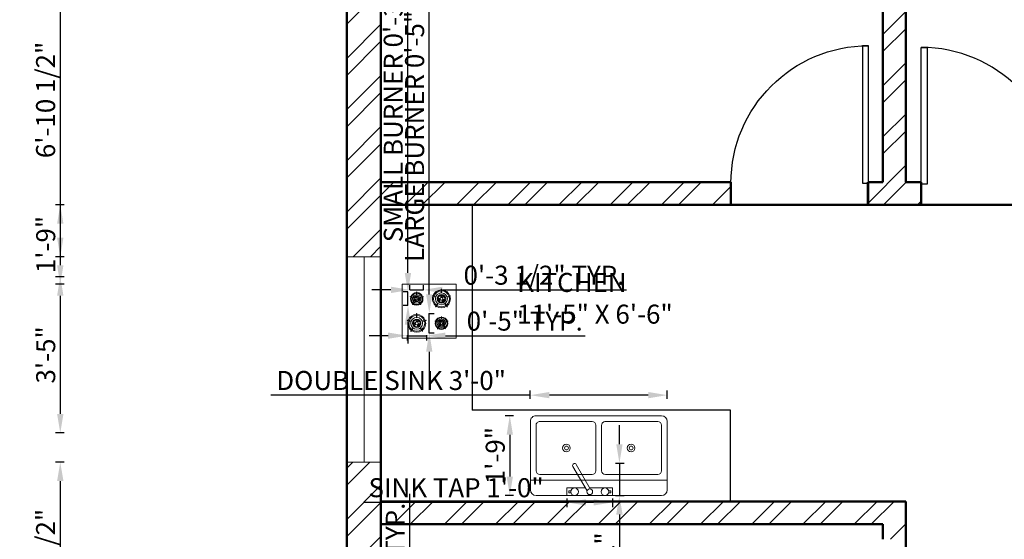
# Model space of a CAD drawing. Units: inches. Extents: x -83 to 371, y -457 to 76.
# Tile 2 of 4: x -83 to 176, y -243 to -107. Entities that reach past the tile are written whole.
import ezdxf

# ---------------------------------------------------------------- set-up
doc = ezdxf.new("R2010")
doc.units = ezdxf.units.IN
for name, color, linetype, lineweight in [('A-ANNO-DIMS', 2, 'Continuous', 18), ('A-AREA-IDEN', 7, 'Continuous', 25), ('A-DOOR', 3, 'Continuous', 25), ('A-EQPM', 8, 'Continuous', 18), ('A-FLOR-CASE', 8, 'Continuous', 25), ('A-FLOR-FIXT', 9, 'Continuous', 18), ('A-GLAZ', 4, 'Continuous', 18), ('A-WALL', 7, 'Continuous', 50), ('A-WALL-PATT', 252, 'Continuous', 13)]:
    doc.layers.add(name, color=color, linetype=linetype, lineweight=lineweight)
doc.styles.get("Standard").update_dxf_attribs({"font": 'arial.ttf'})
doc.dimstyles.new('ISO-25', dxfattribs={"dimtxt": 5, "dimasz": 5, "dimexe": 1.25, "dimexo": 0.625, "dimtad": 1, "dimlunit": 3, "dimtxsty": 'Standard', "dimcen": 2.5, "dimadec": 0, "dimazin": 0, "dimtfac": 1, "dimtmove": 0, "dimatfit": 3, "dimfxl": 1, "dimfxlon": 1, "dimarcsym": 0})

# ---------------------------------------------------------------- blocks, each defined once
blk = doc.blocks.new('*U4')
for p, q in [((0, 0), (0, -6)), ((40, 0), (40, -6))]:
    blk.add_line(p, q)
blk.add_lwpolyline([(0, 0), (0, 40), (1.75, 40), (1.75, 0)], close=True)
blk.add_arc((0, 0), 40, 0, 90)
blk = doc.blocks.new('Sink-double - 36 in top')
for p, q in [((-18, -4), (18, -4)), ((-0.75, -18.5), (-0.75, -6.5)), ((0.75, -6.5), (0.75, -18.5))]:
    blk.add_line(p, q)
for points in [[(-16.5, 0), (16.5, 0)], [(-18, -19.5), (-18, -1.5)], [(18, -1.5), (18, -19.5)], [(-16.5, -18.5), (-16.5, -6.5)], [(-15.5, -5.5), (-1.75, -5.5)], [(1.75, -5.5), (15.5, -5.5)], [(16.5, -6.5), (16.5, -18.5)], [(-1.75, -19.5), (-15.5, -19.5)], [(15.5, -19.5), (1.75, -19.5)], [(16.5, -21), (-16.5, -21)]]:
    blk.add_lwpolyline(points)
for centre, radius in [((-8.5, -12.5), 1), ((-8.5, -12.5), 0.5), ((8.5, -12.5), 1), ((8.5, -12.5), 0.5)]:
    blk.add_circle(centre, radius)
for centre, radius, start, end in [((-16.5, -1.5), 1.5, 90, 180), ((16.5, -1.5), 1.5, 0, 90), ((-15.5, -6.5), 1, 90, 180), ((-1.75, -6.5), 1, 0, 90), ((1.75, -6.5), 1, 90, 180), ((15.5, -6.5), 1, 0, 90), ((-16.5, -19.5), 1.5, 180, 270), ((-15.5, -18.5), 1, 180, 270), ((-1.75, -18.5), 1, 270, 0), ((1.75, -18.5), 1, 180, 270), ((15.5, -18.5), 1, 270, 0), ((16.5, -19.5), 1.5, 270, 0)]:
    blk.add_arc(centre, radius, start, end)
blk = doc.blocks.new('Faucet - kit sink top')
for p, q in [((-5.5, -0.75), (-5.5, -1.25)), ((-4.94278, -0.75), (-5.5, -0.75)), ((-5.5, -1.25), (-4.94278, -1.25)), ((-0.14775, -1.7441), (3.56698, -8.1782)), ((4.43301, -7.6782), (0.71828, -1.2441)), ((4.94278, -0.75), (5.5, -0.75)), ((5.5, -1.25), (4.94278, -1.25)), ((5.5, -0.75), (5.5, -1.25))]:
    blk.add_line(p, q)
blk.add_lwpolyline([(-0.00587, -2), (-6, -2), (-6, 0), (6, 0), (6, -2), (1.15195, -2)])
for centre, radius in [((-4, -1), 1), ((4, -1), 1), ((0, -1), 0.75)]:
    blk.add_circle(centre, radius)
blk.add_arc((4, -7.9282), 0.5, 210, 30)
blk = doc.blocks.new('WIN-54IN')
blk.add_line((4.5, 54), (4.5, 0))
blk.add_lwpolyline([(0, 54), (9, 54), (9, 0), (0, 0)], close=True)
blk = doc.blocks.new('COOKTOP-BURNER-LARGE')
for p, q in [((0.94, 2.8), (0.03, 3.1)), ((0.97, 2.88), (0.05, 3.18)), ((2.44, 3.95), (2.44, 4.91)), ((2.52, 3.95), (2.52, 4.91)), ((3.99, 2.88), (4.91, 3.18)), ((4.02, 2.8), (4.93, 3.1)), ((1.51, 1.07), (0.94, 0.29)), ((1.57, 1.03), (1, 0.25)), ((3.39, 1.03), (3.96, 0.25)), ((3.45, 1.07), (4.02, 0.29))]:
    blk.add_line(p, q)
for radius in [1.56, 1.12, 0.912, 0.391]:
    blk.add_circle((2.48, 2.35), radius)
for centre, radius, start, end in [((0.04, 3.14), 0.0391, 72.0007, 252.0007), ((2.48, 2.35), 2.35, 162.9557, 233.0457), ((2.48, 2.35), 2.35, 90.9557, 161.0457), ((2.48, 2.35), 2.09, 163.075, 232.9263), ((2.48, 2.35), 2.09, 91.075, 160.9263), ((0.95, 2.84), 0.0391, 252.0007, 72.0007), ((2.44, 3), 0.13, 93.5265, 273.5265), ((2.48, 2.35), 0.782, 60.0007, 93.5265), ((2.48, 4.91), 0.0391, 0.0007, 180.0007), ((2.48, 3.95), 0.0391, 180.0007, 0.0007), ((2.48, 2.35), 0.521, 60.0007, 93.5265), ((2.48, 2.35), 2.35, 18.9557, 89.0457), ((2.48, 2.35), 2.09, 19.075, 88.9263), ((2.81, 2.91), 0.13, 240.0007, 60.0007), ((2.48, 2.35), 2.09, 307.075, 16.9263), ((2.48, 2.35), 2.35, 306.9557, 17.0457), ((4, 2.84), 0.0391, 108.0007, 288.0007), ((4.92, 3.14), 0.0391, 288.0007, 108.0007), ((0.97, 0.27), 0.0391, 144.0007, 324.0007), ((2.48, 2.35), 2.35, 234.9557, 305.0457), ((2.48, 2.35), 2.09, 235.075, 304.9263), ((1.54, 1.05), 0.0391, 324.0007, 144.0007), ((1.83, 2.35), 0.13, 0.0007, 180.0007), ((2.48, 2.35), 0.782, 180.0007, 213.5265), ((1.94, 1.99), 0.13, 213.5265, 33.5265), ((2.48, 2.35), 0.521, 180.0007, 213.5265), ((2.81, 1.78), 0.13, 120.0007, 300.0007), ((2.48, 2.35), 0.521, 300.0007, 333.5265), ((2.48, 2.35), 0.782, 300.0007, 333.5265), ((3.06, 2.06), 0.13, 333.5265, 153.5265), ((3.42, 1.05), 0.0391, 36.0007, 216.0007), ((3.99, 0.27), 0.0391, 216.0007, 36.0007)]:
    blk.add_arc(centre, radius, start, end)
blk = doc.blocks.new('COOKTOP-BURNER-SMALL')
for p, q in [((1.71, 2.77), (1.71, 3.44)), ((1.76, 2.77), (1.76, 3.44)), ((0.66, 1.96), (0.02, 2.17)), ((0.68, 2.02), (0.04, 2.22)), ((1.05, 0.75), (0.66, 0.21)), ((1.1, 0.72), (0.7, 0.17)), ((2.37, 0.72), (2.77, 0.17)), ((2.42, 0.75), (2.81, 0.21)), ((2.79, 2.02), (3.44, 2.22)), ((2.81, 1.96), (3.45, 2.17))]:
    blk.add_line(p, q)
for radius in [1.09, 0.785, 0.639, 0.274]:
    blk.add_circle((1.74, 1.64), radius)
for centre, radius, start, end in [((1.74, 1.64), 1.64, 90.9557, 161.0457), ((1.74, 1.64), 1.46, 91.075, 160.9263), ((1.74, 3.44), 0.0274, 0.0007, 180.0007), ((1.74, 2.77), 0.0274, 180.0007, 0.0007), ((1.74, 1.64), 1.64, 18.9557, 89.0457), ((1.74, 1.64), 1.46, 19.075, 88.9263), ((0.03, 2.2), 0.0274, 72.0007, 252.0007), ((1.74, 1.64), 1.64, 162.9557, 233.0457), ((1.74, 1.64), 1.46, 163.075, 232.9263), ((0.68, 0.19), 0.0274, 144.0007, 324.0007), ((0.67, 1.99), 0.0274, 252.0007, 72.0007), ((1.67, 1.64), 1.64, 234.9557, 305.0457), ((1.74, 1.64), 1.46, 235.075, 304.9263), ((1.08, 0.73), 0.0274, 324.0007, 144.0007), ((1.33, 1.44), 0.0912, 26.4748, 206.4748), ((1.74, 1.64), 0.547, 206.4748, 240.0007), ((1.74, 1.64), 0.365, 206.4748, 240.0007), ((1.51, 2.04), 0.0912, 120.0007, 300.0007), ((1.74, 1.64), 0.547, 86.4748, 120.0007), ((1.51, 1.25), 0.0912, 240.0007, 60.0007), ((1.74, 1.64), 0.365, 86.4748, 120.0007), ((1.76, 2.1), 0.0912, 266.4748, 86.4748), ((2.12, 1.39), 0.0912, 146.4748, 326.4748), ((1.74, 1.64), 0.365, 326.4748, 0.0007), ((2.19, 1.64), 0.0912, 0.0007, 180.0007), ((1.74, 1.64), 0.547, 326.4748, 0.0007), ((2.4, 0.73), 0.0274, 36.0007, 216.0007), ((1.74, 1.64), 1.46, 307.075, 16.9263), ((1.74, 1.64), 1.64, 306.9557, 17.0457), ((2.79, 0.19), 0.0274, 216.0007, 36.0007), ((2.8, 1.99), 0.0274, 108.0007, 288.0007), ((3.44, 2.2), 0.0274, 288.0007, 108.0007)]:
    blk.add_arc(centre, radius, start, end)
blk = doc.blocks.new('*D24')
at = {"layer": 'A-ANNO-DIMS', "color": 0, "lineweight": -2, "transparency": 16777216}
for p, q in [((19.57, -332.63), (19.57, -231.32)), ((20.57, -332.63), (18.32, -332.63)), ((19.57, -344.37), (19.57, -337.63)), ((20.57, -349.37), (18.32, -349.37))]:
    blk.add_line(p, q, dxfattribs=at)
at = {"layer": 'A-ANNO-DIMS', "color": 0, "transparency": 16777216}
for points in [[(18.74, -337.63), (20.4, -337.63), (19.57, -332.63)], [(18.74, -344.37), (20.4, -344.37), (19.57, -349.37)]]:
    blk.add_solid(points, dxfattribs=at)
at = {"layer": 'Defpoints', "color": 0, "transparency": 16777216}
for p in [(19.57, -332.63), (22.08, -332.63), (22.08, -349.37)]:
    blk.add_point(p, dxfattribs=at)
at = {"layer": 'A-ANNO-DIMS', "color": 0, "transparency": 16777216, "insert": (16.36, -279.48), "char_height": 5, "attachment_point": 5, "rotation": 90}
blk.add_mtext('NIGHTSTAND L 1\'-4 1/2" TYP.', dxfattribs=at)
blk = doc.blocks.new('*D30')
at = {"layer": 'A-ANNO-DIMS', "color": 0, "lineweight": -2, "transparency": 16777216}
for p, q in [((24.67, -178.88), (24.67, -85.32)), ((24.53, -183.88), (25.92, -183.88)), ((24.67, -188.98), (24.67, -183.88)), ((24.53, -188.98), (25.92, -188.98)), ((24.67, -193.98), (24.67, -198.98))]:
    blk.add_line(p, q, dxfattribs=at)
at = {"layer": 'A-ANNO-DIMS', "color": 0, "transparency": 16777216}
for points in [[(23.83, -178.88), (25.5, -178.88), (24.67, -183.88)], [(23.83, -193.98), (25.5, -193.98), (24.67, -188.98)]]:
    blk.add_solid(points, dxfattribs=at)
at = {"layer": 'Defpoints', "color": 0, "transparency": 16777216}
for p in [(23.9, -183.88), (24.67, -183.88), (23.9, -188.98)]:
    blk.add_point(p, dxfattribs=at)
at = {"layer": 'A-ANNO-DIMS', "color": 0, "transparency": 16777216, "insert": (21.46, -129.6), "char_height": 5, "attachment_point": 5, "rotation": 90}
blk.add_mtext('LARGE BURNER 0\'-5" TYP.', dxfattribs=at)
blk = doc.blocks.new('*D31')
at = {"layer": 'A-ANNO-DIMS', "color": 0, "lineweight": -2, "transparency": 16777216}
for p, q in [((13.84, -189.74), (8.84, -189.74)), ((18.84, -189.6), (18.84, -190.99)), ((18.84, -189.74), (23.9, -189.74)), ((23.9, -189.6), (23.9, -190.99)), ((28.9, -189.74), (65.63, -189.74))]:
    blk.add_line(p, q, dxfattribs=at)
at = {"layer": 'A-ANNO-DIMS', "color": 0, "transparency": 16777216}
for points in [[(13.84, -188.91), (13.84, -190.57), (18.84, -189.74)], [(28.9, -188.91), (28.9, -190.57), (23.9, -189.74)]]:
    blk.add_solid(points, dxfattribs=at)
at = {"layer": 'Defpoints', "color": 0, "transparency": 16777216}
for p in [(18.84, -188.98), (23.9, -188.98), (23.9, -189.74)]:
    blk.add_point(p, dxfattribs=at)
at = {"layer": 'A-ANNO-DIMS', "color": 0, "transparency": 16777216, "insert": (49.77, -186.56), "char_height": 5, "attachment_point": 5}
blk.add_mtext('0\'-5" TYP.', dxfattribs=at)
blk = doc.blocks.new('*D32')
at = {"layer": 'A-ANNO-DIMS', "color": 0, "lineweight": -2, "transparency": 16777216}
for p, q in [((19.06, -173.23), (19.06, -68.59)), ((19.06, -178.23), (17.81, -178.23)), ((19.06, -181.8), (19.06, -178.23)), ((19.06, -181.8), (17.81, -181.8)), ((19.06, -186.8), (19.06, -191.8))]:
    blk.add_line(p, q, dxfattribs=at)
at = {"layer": 'A-ANNO-DIMS', "color": 0, "transparency": 16777216}
for points in [[(18.23, -173.23), (19.9, -173.23), (19.06, -178.23)], [(18.23, -186.8), (19.9, -186.8), (19.06, -181.8)]]:
    blk.add_solid(points, dxfattribs=at)
at = {"layer": 'Defpoints', "color": 0, "transparency": 16777216}
for p in [(19.06, -178.23), (19.6, -178.23), (19.6, -181.8)]:
    blk.add_point(p, dxfattribs=at)
at = {"layer": 'A-ANNO-DIMS', "color": 0, "transparency": 16777216, "insert": (15.85, -118.41), "char_height": 5, "attachment_point": 5, "rotation": 90}
blk.add_mtext('SMALL BURNER 0\'-3 1/2" TYP.', dxfattribs=at)
blk = doc.blocks.new('*D33')
at = {"layer": 'A-ANNO-DIMS', "color": 0, "lineweight": -2, "transparency": 16777216}
for p, q in [((14.6, -177.7), (9.6, -177.7)), ((19.6, -177.7), (19.6, -176.45)), ((19.6, -177.7), (23.14, -177.7)), ((23.14, -177.7), (23.14, -176.45)), ((28.14, -177.7), (76.52, -177.7))]:
    blk.add_line(p, q, dxfattribs=at)
at = {"layer": 'A-ANNO-DIMS', "color": 0, "transparency": 16777216}
for points in [[(14.6, -176.86), (14.6, -178.53), (19.6, -177.7)], [(28.14, -176.86), (28.14, -178.53), (23.14, -177.7)]]:
    blk.add_solid(points, dxfattribs=at)
at = {"layer": 'Defpoints', "color": 0, "transparency": 16777216}
for p in [(19.6, -178.23), (23.14, -177.7), (23.14, -178.23)]:
    blk.add_point(p, dxfattribs=at)
at = {"layer": 'A-ANNO-DIMS', "color": 0, "transparency": 16777216, "insert": (54.83, -174.48), "char_height": 5, "attachment_point": 5}
blk.add_mtext('0\'-3 1/2" TYP.', dxfattribs=at)
blk = doc.blocks.new('*D34')
at = {"layer": 'A-ANNO-DIMS', "color": 0, "lineweight": -2, "transparency": 16777216}
for p, q in [((51.24, -206.38), (51.24, -204.13)), ((87.24, -206.38), (87.24, -204.13)), ((51.24, -205.38), (-16.96, -205.38)), ((82.24, -205.38), (56.24, -205.38))]:
    blk.add_line(p, q, dxfattribs=at)
at = {"layer": 'A-ANNO-DIMS', "color": 0, "transparency": 16777216}
for points in [[(56.24, -204.55), (56.24, -206.21), (51.24, -205.38)], [(82.24, -204.55), (82.24, -206.21), (87.24, -205.38)]]:
    blk.add_solid(points, dxfattribs=at)
at = {"layer": 'Defpoints', "color": 0, "transparency": 16777216}
for p in [(51.24, -205.38), (51.24, -210.78), (87.24, -210.78)]:
    blk.add_point(p, dxfattribs=at)
at = {"layer": 'A-ANNO-DIMS', "color": 0, "transparency": 16777216, "insert": (14.64, -202.17), "char_height": 5, "attachment_point": 5}
blk.add_mtext('DOUBLE SINK 3\'-0"', dxfattribs=at)
blk = doc.blocks.new('*D35')
at = {"layer": 'A-ANNO-DIMS', "color": 0, "lineweight": -2, "transparency": 16777216}
for p, q in [((46.84, -210.78), (44.59, -210.78)), ((45.84, -215.78), (45.84, -226.78)), ((46.84, -231.78), (44.59, -231.78))]:
    blk.add_line(p, q, dxfattribs=at)
at = {"layer": 'A-ANNO-DIMS', "color": 0, "transparency": 16777216}
for points in [[(45.01, -215.78), (46.67, -215.78), (45.84, -210.78)], [(45.01, -226.78), (46.67, -226.78), (45.84, -231.78)]]:
    blk.add_solid(points, dxfattribs=at)
at = {"layer": 'Defpoints', "color": 0, "transparency": 16777216}
for p in [(51.24, -210.78), (45.84, -231.78), (51.24, -231.78)]:
    blk.add_point(p, dxfattribs=at)
at = {"layer": 'A-ANNO-DIMS', "color": 0, "transparency": 16777216, "insert": (42.66, -221.28), "char_height": 5, "attachment_point": 5, "rotation": 90}
blk.add_mtext('1\'-9"', dxfattribs=at)
blk = doc.blocks.new('*D36')
at = {"layer": 'A-ANNO-DIMS', "color": 0, "lineweight": -2, "transparency": 16777216}
for p, q in [((60.86, -232.58), (60.86, -234.83)), ((72.86, -232.58), (72.86, -234.83)), ((60.86, -233.58), (7.58, -233.58)), ((67.86, -233.58), (65.86, -233.58))]:
    blk.add_line(p, q, dxfattribs=at)
at = {"layer": 'A-ANNO-DIMS', "color": 0, "transparency": 16777216}
for points in [[(65.86, -232.75), (65.86, -234.41), (60.86, -233.58)], [(67.86, -232.75), (67.86, -234.41), (72.86, -233.58)]]:
    blk.add_solid(points, dxfattribs=at)
at = {"layer": 'Defpoints', "color": 0, "transparency": 16777216}
for p in [(60.86, -231.78), (72.86, -231.78), (60.86, -233.58)]:
    blk.add_point(p, dxfattribs=at)
at = {"layer": 'A-ANNO-DIMS', "color": 0, "transparency": 16777216, "insert": (31.72, -230.37), "char_height": 5, "attachment_point": 5}
blk.add_mtext('SINK TAP 1\'-0"', dxfattribs=at)
blk = doc.blocks.new('*D37')
at = {"layer": 'A-ANNO-DIMS', "color": 0, "lineweight": -2, "transparency": 16777216}
for p, q in [((74.66, -218.28), (74.66, -213.28)), ((73.66, -223.28), (75.91, -223.28)), ((74.66, -223.28), (74.66, -231.78)), ((73.66, -231.78), (75.91, -231.78)), ((74.66, -236.78), (74.66, -267.97))]:
    blk.add_line(p, q, dxfattribs=at)
at = {"layer": 'A-ANNO-DIMS', "color": 0, "transparency": 16777216}
for points in [[(73.83, -218.28), (75.5, -218.28), (74.66, -223.28)], [(73.83, -236.78), (75.5, -236.78), (74.66, -231.78)]]:
    blk.add_solid(points, dxfattribs=at)
at = {"layer": 'Defpoints', "color": 0, "transparency": 16777216}
for p in [(72.86, -223.28), (72.86, -231.78), (74.66, -231.78)]:
    blk.add_point(p, dxfattribs=at)
at = {"layer": 'A-ANNO-DIMS', "color": 0, "transparency": 16777216, "insert": (71.45, -254.88), "char_height": 5, "attachment_point": 5, "rotation": 90}
blk.add_mtext('0\'-8 1/2"', dxfattribs=at)
blk = doc.blocks.new('*D39')
at = {"layer": 'A-ANNO-DIMS', "color": 0, "lineweight": -2, "transparency": 16777216}
for p, q in [((-71.36, -86.5), (-73.61, -86.5)), ((-72.36, -91.5), (-72.36, -163.99)), ((-71.36, -168.99), (-73.61, -168.99))]:
    blk.add_line(p, q, dxfattribs=at)
at = {"layer": 'A-ANNO-DIMS', "color": 0, "transparency": 16777216}
for points in [[(-73.19, -91.5), (-71.52, -91.5), (-72.36, -86.5)], [(-73.19, -163.99), (-71.52, -163.99), (-72.36, -168.99)]]:
    blk.add_solid(points, dxfattribs=at)
at = {"layer": 'Defpoints', "color": 0, "transparency": 16777216}
for p in [(2.94, -86.5), (-72.36, -168.99), (3.06, -168.99)]:
    blk.add_point(p, dxfattribs=at)
at = {"layer": 'A-ANNO-DIMS', "color": 0, "transparency": 16777216, "insert": (-75.57, -127.74), "char_height": 5, "attachment_point": 5, "rotation": 90}
blk.add_mtext('6\'-10 1/2"', dxfattribs=at)
blk = doc.blocks.new('*D40')
at = {"layer": 'A-ANNO-DIMS', "color": 0, "lineweight": -2, "transparency": 16777216}
for p, q in [((-71.36, -222.99), (-73.61, -222.99)), ((-72.36, -227.99), (-72.36, -269.39)), ((-71.36, -274.39), (-73.61, -274.39))]:
    blk.add_line(p, q, dxfattribs=at)
at = {"layer": 'A-ANNO-DIMS', "color": 0, "transparency": 16777216}
for points in [[(-73.19, -227.99), (-71.52, -227.99), (-72.36, -222.99)], [(-73.19, -269.39), (-71.52, -269.39), (-72.36, -274.39)]]:
    blk.add_solid(points, dxfattribs=at)
at = {"layer": 'Defpoints', "color": 0, "transparency": 16777216}
for p in [(3.06, -222.99), (-72.36, -274.39), (3.85, -274.39)]:
    blk.add_point(p, dxfattribs=at)
at = {"layer": 'A-ANNO-DIMS', "color": 0, "transparency": 16777216, "insert": (-75.57, -248.69), "char_height": 5, "attachment_point": 5, "rotation": 90}
blk.add_mtext('4\'-3 1/2"', dxfattribs=at)
blk = doc.blocks.new('*D45')
at = {"layer": 'A-ANNO-DIMS', "color": 0, "lineweight": -2, "transparency": 16777216}
for p, q in [((143.97, -455.2), (143.97, -457.45)), ((149.97, -455.2), (149.97, -457.45)), ((138.97, -456.2), (133.97, -456.2)), ((143.97, -456.2), (149.97, -456.2)), ((154.97, -456.2), (174.51, -456.2))]:
    blk.add_line(p, q, dxfattribs=at)
at = {"layer": 'A-ANNO-DIMS', "color": 0, "transparency": 16777216}
for points in [[(138.97, -455.37), (138.97, -457.03), (143.97, -456.2)], [(154.97, -455.37), (154.97, -457.03), (149.97, -456.2)]]:
    blk.add_solid(points, dxfattribs=at)
at = {"layer": 'Defpoints', "color": 0, "transparency": 16777216}
for p in [(143.97, 6.68), (149.97, 6.68), (149.97, -456.2)]:
    blk.add_point(p, dxfattribs=at)
at = {"layer": 'A-ANNO-DIMS', "color": 0, "transparency": 16777216, "insert": (167.24, -453.02), "char_height": 5, "attachment_point": 5}
blk.add_mtext('0\'-6"', dxfattribs=at)
blk = doc.blocks.new('*D46')
at = {"layer": 'A-ANNO-DIMS', "color": 0, "lineweight": -2, "transparency": 16777216}
for p, q in [((103.97, 39.58), (103.97, 41.83)), ((139.97, 39.58), (139.97, 41.83)), ((108.97, 40.58), (134.97, 40.58))]:
    blk.add_line(p, q, dxfattribs=at)
at = {"layer": 'A-ANNO-DIMS', "color": 0, "transparency": 16777216}
for points in [[(108.97, 41.41), (108.97, 39.74), (103.97, 40.58)], [(134.97, 41.41), (134.97, 39.74), (139.97, 40.58)]]:
    blk.add_solid(points, dxfattribs=at)
at = {"layer": 'Defpoints', "color": 0, "transparency": 16777216}
for p in [(139.97, 40.58), (103.97, -149.32), (139.97, -149.32)]:
    blk.add_point(p, dxfattribs=at)
at = {"layer": 'A-ANNO-DIMS', "color": 0, "transparency": 16777216, "insert": (121.97, 43.75), "char_height": 5, "attachment_point": 5}
blk.add_mtext('3\'-0"', dxfattribs=at)
blk = doc.blocks.new('*D47')
at = {"layer": 'A-ANNO-DIMS', "color": 0, "lineweight": -2, "transparency": 16777216}
for p, q in [((139.97, 39.58), (139.97, 41.83)), ((143.97, 39.58), (143.97, 41.83)), ((134.97, 40.58), (129.97, 40.58)), ((139.97, 40.58), (143.97, 40.58)), ((148.97, 40.58), (168.51, 40.58))]:
    blk.add_line(p, q, dxfattribs=at)
at = {"layer": 'A-ANNO-DIMS', "color": 0, "transparency": 16777216}
for points in [[(134.97, 41.41), (134.97, 39.74), (139.97, 40.58)], [(148.97, 41.41), (148.97, 39.74), (143.97, 40.58)]]:
    blk.add_solid(points, dxfattribs=at)
at = {"layer": 'Defpoints', "color": 0, "transparency": 16777216}
for p in [(143.97, 40.58), (139.97, -149.32), (143.97, -149.32)]:
    blk.add_point(p, dxfattribs=at)
at = {"layer": 'A-ANNO-DIMS', "color": 0, "transparency": 16777216, "insert": (161.24, 43.75), "char_height": 5, "attachment_point": 5}
blk.add_mtext('0\'-4"', dxfattribs=at)
blk = doc.blocks.new('*D55')
at = {"layer": 'A-ANNO-DIMS', "color": 0, "lineweight": -2, "transparency": 16777216}
for p, q in [((11.97, -455.2), (11.97, -457.45)), ((103.87, -455.2), (103.87, -457.45)), ((16.97, -456.2), (98.87, -456.2))]:
    blk.add_line(p, q, dxfattribs=at)
at = {"layer": 'A-ANNO-DIMS', "color": 0, "transparency": 16777216}
for points in [[(16.97, -455.37), (16.97, -457.03), (11.97, -456.2)], [(98.87, -455.37), (98.87, -457.03), (103.87, -456.2)]]:
    blk.add_solid(points, dxfattribs=at)
at = {"layer": 'Defpoints', "color": 0, "transparency": 16777216}
for p in [(11.97, -233.32), (103.87, -233.32), (103.87, -456.2)]:
    blk.add_point(p, dxfattribs=at)
at = {"layer": 'A-ANNO-DIMS', "color": 0, "transparency": 16777216, "insert": (57.92, -453.02), "char_height": 5, "attachment_point": 5}
blk.add_mtext('7\'-8"', dxfattribs=at)
blk = doc.blocks.new('*D56')
at = {"layer": 'A-ANNO-DIMS', "color": 0, "lineweight": -2, "transparency": 16777216}
for p, q in [((365.66, -209.32), (367.91, -209.32)), ((366.66, -228.32), (366.66, -214.32)), ((365.66, -233.32), (367.91, -233.32))]:
    blk.add_line(p, q, dxfattribs=at)
at = {"layer": 'A-ANNO-DIMS', "color": 0, "transparency": 16777216}
for points in [[(365.83, -214.32), (367.49, -214.32), (366.66, -209.32)], [(365.83, -228.32), (367.49, -228.32), (366.66, -233.32)]]:
    blk.add_solid(points, dxfattribs=at)
at = {"layer": 'Defpoints', "color": 0, "transparency": 16777216}
for p in [(103.87, -209.32), (366.66, -209.32), (103.87, -233.32)]:
    blk.add_point(p, dxfattribs=at)
at = {"layer": 'A-ANNO-DIMS', "color": 0, "transparency": 16777216, "insert": (363.48, -221.32), "char_height": 5, "attachment_point": 5, "rotation": 90}
blk.add_mtext('2\'-0"', dxfattribs=at)
blk = doc.blocks.new('*D57')
at = {"layer": 'A-ANNO-DIMS', "color": 0, "lineweight": -2, "transparency": 16777216}
for p, q in [((365.66, -155.32), (367.91, -155.32)), ((366.66, -160.32), (366.66, -204.32)), ((365.66, -209.32), (367.91, -209.32))]:
    blk.add_line(p, q, dxfattribs=at)
at = {"layer": 'A-ANNO-DIMS', "color": 0, "transparency": 16777216}
for points in [[(365.83, -160.32), (367.49, -160.32), (366.66, -155.32)], [(365.83, -204.32), (367.49, -204.32), (366.66, -209.32)]]:
    blk.add_solid(points, dxfattribs=at)
at = {"layer": 'Defpoints', "color": 0, "transparency": 16777216}
for p in [(35.97, -155.32), (35.97, -209.32), (366.66, -209.32)]:
    blk.add_point(p, dxfattribs=at)
at = {"layer": 'A-ANNO-DIMS', "color": 0, "transparency": 16777216, "insert": (363.48, -182.32), "char_height": 5, "attachment_point": 5, "rotation": 90}
blk.add_mtext('4\'-6"', dxfattribs=at)
blk = doc.blocks.new('*D58')
at = {"layer": 'A-ANNO-DIMS', "color": 0, "lineweight": -2, "transparency": 16777216}
for p, q in [((11.97, 39.58), (11.97, 41.83)), ((35.97, 39.58), (35.97, 41.83)), ((16.97, 40.58), (30.97, 40.58))]:
    blk.add_line(p, q, dxfattribs=at)
at = {"layer": 'A-ANNO-DIMS', "color": 0, "transparency": 16777216}
for points in [[(16.97, 41.41), (16.97, 39.74), (11.97, 40.58)], [(30.97, 41.41), (30.97, 39.74), (35.97, 40.58)]]:
    blk.add_solid(points, dxfattribs=at)
at = {"layer": 'Defpoints', "color": 0, "transparency": 16777216}
for p in [(35.97, 40.58), (11.97, -155.32), (35.97, -155.32)]:
    blk.add_point(p, dxfattribs=at)
at = {"layer": 'A-ANNO-DIMS', "color": 0, "transparency": 16777216, "insert": (23.97, 43.75), "char_height": 5, "attachment_point": 5}
blk.add_mtext('2\'-0"', dxfattribs=at)
blk = doc.blocks.new('*D59')
at = {"layer": 'A-ANNO-DIMS', "color": 0, "lineweight": -2, "transparency": 16777216}
for p, q in [((17.51, 39.58), (17.51, 41.83)), ((31.73, 39.58), (31.73, 41.83)), ((22.51, 40.58), (26.73, 40.58))]:
    blk.add_line(p, q, dxfattribs=at)
at = {"layer": 'A-ANNO-DIMS', "color": 0, "transparency": 16777216}
for points in [[(22.51, 41.41), (22.51, 39.74), (17.51, 40.58)], [(26.73, 41.41), (26.73, 39.74), (31.73, 40.58)]]:
    blk.add_solid(points, dxfattribs=at)
at = {"layer": 'Defpoints', "color": 0, "transparency": 16777216}
for p in [(31.73, 40.58), (17.51, -176.2), (31.73, -176.2)]:
    blk.add_point(p, dxfattribs=at)
at = {"layer": 'A-ANNO-DIMS', "color": 0, "transparency": 16777216, "insert": (24.62, 43.71), "char_height": 5, "attachment_point": 5}
blk.add_mtext('1\'-2"', dxfattribs=at)
blk = doc.blocks.new('*D60')
at = {"layer": 'A-ANNO-DIMS', "color": 0, "lineweight": -2, "transparency": 16777216}
for p, q in [((365.66, -176.2), (367.91, -176.2)), ((366.66, -181.2), (366.66, -185.42)), ((365.66, -190.42), (367.91, -190.42))]:
    blk.add_line(p, q, dxfattribs=at)
at = {"layer": 'A-ANNO-DIMS', "color": 0, "transparency": 16777216}
for points in [[(365.83, -181.2), (367.49, -181.2), (366.66, -176.2)], [(365.83, -185.42), (367.49, -185.42), (366.66, -190.42)]]:
    blk.add_solid(points, dxfattribs=at)
at = {"layer": 'Defpoints', "color": 0, "transparency": 16777216}
for p in [(31.73, -176.2), (31.73, -190.42), (366.66, -190.42)]:
    blk.add_point(p, dxfattribs=at)
at = {"layer": 'A-ANNO-DIMS', "color": 0, "transparency": 16777216, "insert": (363.52, -183.31), "char_height": 5, "attachment_point": 5, "rotation": 90}
blk.add_mtext('1\'-2"', dxfattribs=at)
blk = doc.blocks.new('*D62')
at = {"layer": 'A-ANNO-DIMS', "color": 0, "lineweight": -2, "transparency": 16777216}
for p, q in [((-71.36, -174.24), (-73.61, -174.24)), ((-72.36, -179.24), (-72.36, -210.33)), ((-71.36, -215.33), (-73.61, -215.33))]:
    blk.add_line(p, q, dxfattribs=at)
at = {"layer": 'A-ANNO-DIMS', "color": 0, "transparency": 16777216}
for points in [[(-73.19, -179.24), (-71.52, -179.24), (-72.36, -174.24)], [(-73.19, -210.33), (-71.52, -210.33), (-72.36, -215.33)]]:
    blk.add_solid(points, dxfattribs=at)
at = {"layer": 'Defpoints', "color": 0, "transparency": 16777216}
for p in [(234.88, -174.24), (-72.36, -215.33), (234.88, -215.33)]:
    blk.add_point(p, dxfattribs=at)
at = {"layer": 'A-ANNO-DIMS', "color": 0, "transparency": 16777216, "insert": (-75.54, -194.79), "char_height": 5, "attachment_point": 5, "rotation": 90}
blk.add_mtext('3\'-5"', dxfattribs=at)
blk = doc.blocks.new('*D65')
at = {"layer": 'A-ANNO-DIMS', "color": 0, "lineweight": -2, "transparency": 16777216}
for p, q in [((86.8, 39.58), (86.8, 41.83)), ((103.87, 39.58), (103.87, 41.83)), ((91.8, 40.58), (98.87, 40.58))]:
    blk.add_line(p, q, dxfattribs=at)
at = {"layer": 'A-ANNO-DIMS', "color": 0, "transparency": 16777216}
for points in [[(91.8, 41.41), (91.8, 39.74), (86.8, 40.58)], [(98.87, 41.41), (98.87, 39.74), (103.87, 40.58)]]:
    blk.add_solid(points, dxfattribs=at)
at = {"layer": 'Defpoints', "color": 0, "transparency": 16777216}
for p in [(103.87, 40.58), (103.87, -209.32), (86.8, -211.22)]:
    blk.add_point(p, dxfattribs=at)
at = {"layer": 'A-ANNO-DIMS', "color": 0, "transparency": 16777216, "insert": (95.33, 43.75), "char_height": 5, "attachment_point": 5}
blk.add_mtext('1\'-5"', dxfattribs=at)
blk = doc.blocks.new('*D66')
at = {"layer": 'A-ANNO-DIMS', "color": 0, "lineweight": -2, "transparency": 16777216}
for p, q in [((-71.36, -155.32), (-73.61, -155.32)), ((-72.36, -160.32), (-72.36, -171.2)), ((-71.36, -176.2), (-73.61, -176.2))]:
    blk.add_line(p, q, dxfattribs=at)
at = {"layer": 'A-ANNO-DIMS', "color": 0, "transparency": 16777216}
for points in [[(-73.19, -160.32), (-71.52, -160.32), (-72.36, -155.32)], [(-73.19, -171.2), (-71.52, -171.2), (-72.36, -176.2)]]:
    blk.add_solid(points, dxfattribs=at)
at = {"layer": 'Defpoints', "color": 0, "transparency": 16777216}
for p in [(11.97, -155.32), (-72.36, -176.2), (17.51, -176.2)]:
    blk.add_point(p, dxfattribs=at)
at = {"layer": 'A-ANNO-DIMS', "color": 0, "transparency": 16777216, "insert": (-75.54, -165.76), "char_height": 5, "attachment_point": 5, "rotation": 90}
blk.add_mtext('1\'-9"', dxfattribs=at)
blk = doc.blocks.new('*D67')
at = {"layer": 'A-ANNO-DIMS', "color": 0, "lineweight": -2, "transparency": 16777216}
for p, q in [((11.97, 39.58), (11.97, 41.83)), ((17.51, 39.58), (17.51, 41.83)), ((6.97, 40.58), (1.97, 40.58)), ((11.97, 40.58), (17.51, 40.58)), ((22.51, 40.58), (53.7, 40.58))]:
    blk.add_line(p, q, dxfattribs=at)
at = {"layer": 'A-ANNO-DIMS', "color": 0, "transparency": 16777216}
for points in [[(6.97, 41.41), (6.97, 39.74), (11.97, 40.58)], [(22.51, 41.41), (22.51, 39.74), (17.51, 40.58)]]:
    blk.add_solid(points, dxfattribs=at)
at = {"layer": 'Defpoints', "color": 0, "transparency": 16777216}
for p in [(17.51, 40.58), (11.97, -155.32), (17.51, -176.2)]:
    blk.add_point(p, dxfattribs=at)
at = {"layer": 'A-ANNO-DIMS', "color": 0, "transparency": 16777216, "insert": (40.61, 43.79), "char_height": 5, "attachment_point": 5}
blk.add_mtext('0\'-5 1/2"', dxfattribs=at)

msp = doc.modelspace()

# ---------------------------------------------------------------- hatches: boundary and pattern name
at = {"layer": 'A-WALL-PATT'}
h = msp.add_hatch(dxfattribs=at)
h.set_pattern_fill('ANSI32', color=256)
h.set_pattern_definition([(45, (-445.966, 5e-14), (-6.73519, 6.73519), []), (45, (-441.476, 5e-14), (-6.73519, 6.73519), [])])
h.paths.add_polyline_path([(147.969, -419.325), (11.969, -419.325), (11.969, -408.128), (2.969, -408.128), (2.969, -428.325), (147.969, -428.325)])
h.paths.add_polyline_path([(290.969, -408.128), (281.969, -408.128), (281.969, -419.325), (197.969, -419.325), (197.969, -428.325), (290.969, -428.325)])
h.paths.add_polyline_path([(203.969, -374.325), (207.969, -374.325), (207.969, -368.325), (203.969, -368.325), (203.969, -279.294), (197.969, -279.294), (197.969, -317.37), (194.142, -317.37), (194.142, -317.678), (194.142, -323.37), (197.969, -323.37), (197.969, -374.325), (197.969, -419.325), (203.969, -419.325)])
h.paths.add_polyline_path([(290.969, -249.793), (281.969, -249.793), (281.969, -390.128), (290.969, -390.128)])
h.paths.add_polyline_path([(149.969, -323.37), (157.969, -323.37), (157.969, -317.37), (149.969, -317.37), (149.969, -279.294), (143.969, -279.294), (143.969, -371.325), (140.142, -371.325), (140.142, -371.632), (140.142, -377.325), (143.969, -377.325), (149.969, -377.325)])
h.paths.add_polyline_path([(103.969, -371.325), (11.969, -371.325), (11.969, -377.325), (103.969, -377.325)])
h.paths.add_polyline_path([(11.969, -328.391), (3.855, -328.391), (3.855, -274.391), (11.969, -274.391), (11.969, -222.986), (2.969, -222.986), (2.969, -390.128), (11.969, -390.128)])
h.paths.add_polyline_path([(149.969, -233.325), (143.969, -233.325), (11.969, -233.325), (11.969, -239.325), (143.969, -239.325), (143.969, -243.294), (144.688, -243.294), (149.969, -243.294)])
h.paths.add_polyline_path([(11.969, -86.501), (2.969, -86.501), (2.969, -168.986), (11.969, -168.986)])
h.paths.add_polyline_path([(103.969, -149.325), (11.969, -149.325), (11.969, -155.325), (103.969, -155.325)])
h.paths.add_polyline_path([(149.969, 6.675), (143.969, 6.675), (143.969, -149.325), (139.969, -149.325), (139.969, -155.325), (153.969, -155.325), (153.969, -149.325), (149.969, -149.325)])
h.paths.add_polyline_path([(281.969, -149.325), (189.973, -149.325, -0.0041567), (189.978, -149.923), (189.978, -155.325), (281.969, -155.325)])
h.paths.add_polyline_path([(290.969, -90.886), (281.969, -90.886), (281.969, -195.793), (290.969, -195.793)])
h.paths.add_polyline_path([(290.969, 15.675), (2.969, 15.675), (2.969, -32.501), (11.969, -32.501), (11.969, 6.675), (281.969, 6.675), (281.969, -36.886), (290.969, -36.886)])

# ---------------------------------------------------------------- linework, layer by layer
at = {"layer": 'A-EQPM'}
msp.add_lwpolyline([(17.509, -190.423), (31.729, -190.423), (31.729, -176.204), (17.509, -176.204)], close=True, dxfattribs=at)
at = {"layer": 'A-FLOR-CASE'}
for p, q in [((35.969, -155.325), (35.969, -209.325)), ((103.866, -209.325), (35.969, -209.325)), ((103.866, -233.325), (103.866, -209.325))]:
    msp.add_line(p, q, dxfattribs=at)
at = {"layer": 'A-WALL'}
for p, q in [((2.969, -428.325), (2.969, 15.675)), ((11.969, -419.325), (11.969, 6.675)), ((143.969, -149.325), (143.969, 6.675)), ((149.969, -149.325), (149.969, 6.675)), ((11.969, -149.325), (103.969, -149.325)), ((103.969, -149.325), (103.969, -155.325)), ((139.969, -149.325), (139.969, -155.325)), ((139.969, -149.325), (143.969, -149.325)), ((149.969, -149.325), (153.969, -149.325)), ((153.969, -149.325), (153.969, -155.325)), ((11.969, -155.325), (281.969, -155.325)), ((143.969, -233.325), (11.969, -233.325)), ((143.969, -233.325), (149.969, -233.325)), ((149.969, -317.37), (149.969, -233.325)), ((143.969, -239.325), (11.969, -239.325)), ((143.969, -243.294), (143.969, -239.325))]:
    msp.add_line(p, q, dxfattribs=at)

# ---------------------------------------------------------------- block references
at = {"layer": 'A-DOOR'}
for p, xscale, yscale, zscale in [((140.142, -149.632), -0.9035591955078199, 0.9035591955078199, 0.9035591955078199), ((153.969, -149.923), 0.9002205977698526, 0.9002205977698526, 0.9002205977698526)]:
    msp.add_blockref('*U4', p, dxfattribs=dict(at, xscale=xscale, yscale=yscale, zscale=zscale))
at = {"layer": 'A-EQPM'}
for name, p in [('COOKTOP-BURNER-SMALL', (19.634, -181.698)), ('COOKTOP-BURNER-LARGE', (25.389, -182.401)), ('COOKTOP-BURNER-LARGE', (18.89, -188.833)), ('COOKTOP-BURNER-SMALL', (26.133, -188.13))]:
    msp.add_blockref(name, p, dxfattribs=at)
at = {"layer": 'A-FLOR-FIXT', "rotation": 180}
for name, p in [('Sink-double - 36 in top', (69.241, -231.78)), ('Faucet - kit sink top', (66.863, -231.78))]:
    msp.add_blockref(name, p, dxfattribs=at)
at = {"layer": 'A-GLAZ'}
msp.add_blockref('WIN-54IN', (3.061, -222.986), dxfattribs=at)

# ---------------------------------------------------------------- texts
at = {"layer": 'A-AREA-IDEN', "insert": (47.79, -173.239), "char_height": 5, "attachment_point": 1}
msp.add_mtext_dynamic_manual_height_columns('KITCHEN\\P11\'-5" X 6\'-6"', width=56.40605, gutter_width=12.5, heights=[0], dxfattribs=at)

# ---------------------------------------------------------------- dimensions: what is measured, and where the dimension line sits
at = {"layer": 'A-ANNO-DIMS'}
for base, p1, p2, picture, middle in [((17.509, 40.575), (11.969, -155.325), (17.509, -176.204), '*D67', (40.605, 43.786)), ((35.969, 40.575), (11.969, -155.325), (35.969, -155.325), '*D58', (23.969, 43.753)), ((31.729, 40.575), (17.509, -176.204), (31.729, -176.204), '*D59', (24.619, 43.711)), ((103.866, 40.575), (86.802, -211.219), (103.866, -209.325), '*D65', (95.334, 43.753)), ((139.969, 40.575), (103.969, -149.325), (139.969, -149.325), '*D46', (121.969, 43.755)), ((143.969, 40.575), (139.969, -149.325), (143.969, -149.325), '*D47', (161.24, 43.753)), ((149.969, -456.2), (143.969, 6.675), (149.969, 6.675), '*D45', (167.24, -453.022)), ((103.866, -456.2), (11.969, -233.325), (103.866, -233.325), '*D55', (57.917, -453.022))]:
    dim = msp.add_linear_dim(base=base, p1=p1, p2=p2, dimstyle='ISO-25', override={"dimdec": 1, "dimlfac": 1, "dimrnd": 0, "dimzin": 1, "dimdsep": 46, "dimlunit": 4, "dimfrac": 2}, dxfattribs=at)
    dim.commit()
    dim.dimension.update_dxf_attribs({"geometry": picture, "text_midpoint": middle})
for base, p1, p2, angle, text, picture, middle in [((19.062, -178.232), (19.597, -181.797), (19.597, -178.232), 90, 'SMALL BURNER <> TYP.', '*D32', (15.85, -118.413)), ((24.666, -183.882), (23.902, -188.975), (23.902, -183.882), 90, 'LARGE BURNER <> TYP.', '*D30', (21.456, -129.601)), ((51.241, -205.38), (87.241, -210.78), (51.241, -210.78), 180, 'DOUBLE SINK <>', '*D34', (14.64, -202.166)), ((60.863, -233.58), (72.863, -231.78), (60.863, -231.78), 180, 'SINK TAP <>', '*D36', (31.72, -230.37)), ((19.571, -332.627), (22.083, -349.37), (22.083, -332.627), 90, 'NIGHTSTAND L <> TYP.', '*D24', (16.361, -279.475))]:
    dim = msp.add_linear_dim(base=base, p1=p1, p2=p2, angle=angle, text=text, dimstyle='ISO-25', override={"dimdec": 1, "dimlfac": 1, "dimrnd": 0, "dimzin": 1, "dimdsep": 46, "dimlunit": 4, "dimfrac": 2}, dxfattribs=at)
    dim.commit()
    dim.dimension.update_dxf_attribs({"geometry": picture, "text_midpoint": middle})
for base, p1, p2, angle, picture, middle in [((-72.358, -168.986), (2.939, -86.501), (3.062, -168.986), 90, '*D39', (-75.568, -127.743)), ((-72.358, -176.204), (11.969, -155.325), (17.509, -176.204), 90, '*D66', (-75.536, -165.764)), ((366.659, -209.325), (35.969, -155.325), (35.969, -209.325), 90, '*D57', (363.481, -182.325)), ((-72.358, -215.334), (234.884, -174.24), (234.884, -215.334), 90, '*D62', (-75.538, -194.787)), ((366.659, -190.423), (31.729, -176.204), (31.729, -190.423), 90, '*D60', (363.524, -183.314)), ((366.659, -209.325), (103.866, -233.325), (103.866, -209.325), 90, '*D56', (363.481, -221.325)), ((45.841, -231.78), (51.241, -210.78), (51.241, -231.78), 270, '*D35', (42.663, -221.28)), ((74.663, -231.78), (72.863, -223.281), (72.863, -231.78), 270, '*D37', (71.453, -254.876)), ((-72.358, -274.391), (3.062, -222.986), (3.855, -274.391), 90, '*D40', (-75.57, -248.688))]:
    dim = msp.add_linear_dim(base=base, p1=p1, p2=p2, angle=angle, dimstyle='ISO-25', override={"dimdec": 1, "dimlfac": 1, "dimrnd": 0, "dimzin": 1, "dimdsep": 46, "dimlunit": 4, "dimfrac": 2}, dxfattribs=at)
    dim.commit()
    dim.dimension.update_dxf_attribs({"geometry": picture, "text_midpoint": middle})
for base, p1, p2, picture, middle in [((23.143, -177.697), (19.597, -178.232), (23.143, -178.232), '*D33', (54.832, -174.485)), ((23.902, -189.739), (18.837, -188.975), (23.902, -188.975), '*D31', (49.766, -186.561))]:
    dim = msp.add_linear_dim(base=base, p1=p1, p2=p2, text='<> TYP.', dimstyle='ISO-25', override={"dimdec": 1, "dimlfac": 1, "dimrnd": 0, "dimzin": 1, "dimdsep": 46, "dimlunit": 4, "dimfrac": 2}, dxfattribs=at)
    dim.commit()
    dim.dimension.update_dxf_attribs({"geometry": picture, "text_midpoint": middle})

doc.saveas('drawing.dxf')
